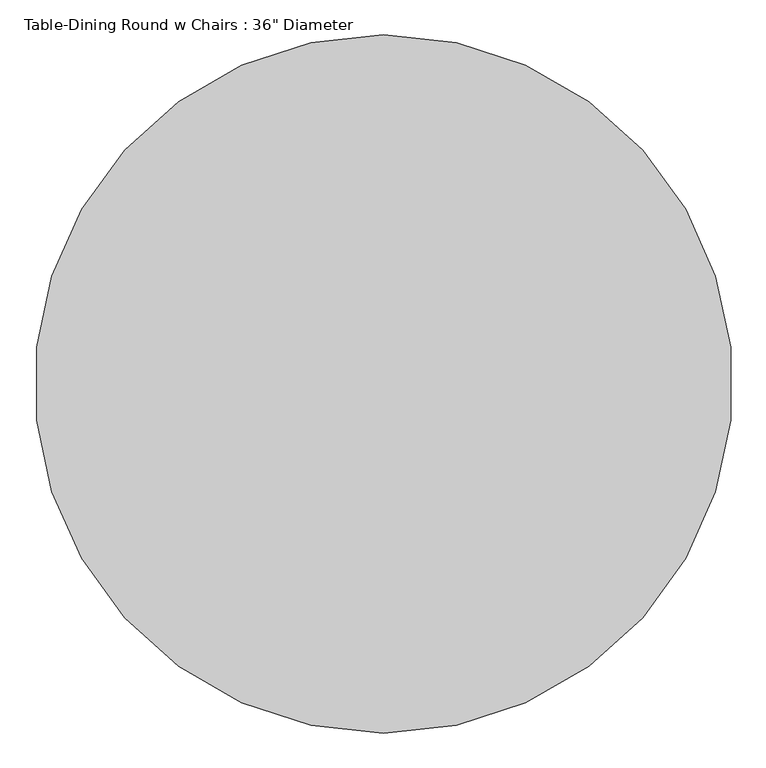
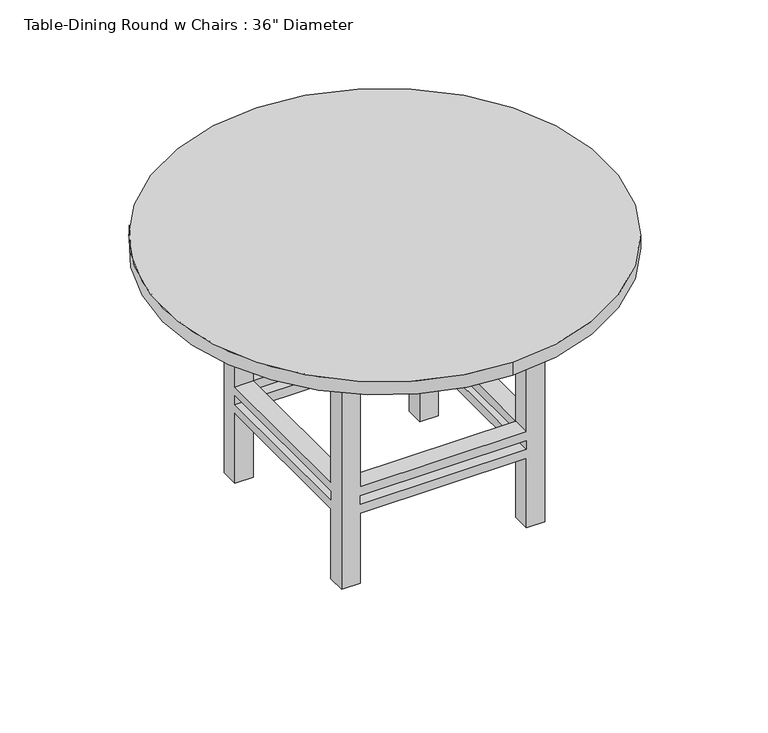
"""IFC4 building model written with IfcOpenShell, lengths in millimetres: furniture geometry."""

from ifc_helpers import new_model, si_unit, point, frame, frame_2d, origin, place, context, project, spatial, polyline, circle_curve, trimmed, segment, composite_curve, outline, extrude, faceted_brep, source, transform, mapped, element, save


def furniture_7060ebe6(model_context):
    return source(origin(), model_context, "Body", "SolidModel", [
        faceted_brep([(332.2819672, 43.7213115, 279.4), (332.2819672, -413.4786885, 279.4), (383.0819672, -413.4786885, 279.4), (383.0819672, 43.7213115, 279.4), (-124.9180328, -413.4786885, 279.4), (-124.9180328, -464.2786885, 279.4), (332.2819672, -464.2786885, 279.4), (-124.9180328, 43.7213115, 279.4), (-175.7180328, 43.7213115, 279.4), (-175.7180328, -413.4786885, 279.4), (332.2819672, 94.5213115, 279.4), (-124.9180328, 94.5213115, 279.4), (332.2819672, 43.7213115, 254.0), (-124.9180328, 43.7213115, 254.0), (-124.9180328, 94.5213115, 254.0), (332.2819672, 94.5213115, 254.0), (-124.9180328, -413.4786885, 254.0), (-175.7180328, -413.4786885, 254.0), (-175.7180328, 43.7213115, 254.0), (332.2819672, -413.4786885, 254.0), (332.2819672, -464.2786885, 254.0), (-124.9180328, -464.2786885, 254.0), (383.0819672, 43.7213115, 254.0), (383.0819672, -413.4786885, 254.0), (-175.7180328, 94.5213115, 647.7), (-124.9180328, 94.5213115, 647.7), (332.2819672, 94.5213115, 647.7), (383.0819672, 94.5213115, 647.7), (383.0819672, 94.5213115, 0.0), (332.2819672, 94.5213115, 0.0), (332.2819672, 94.5213115, 203.2), (-124.9180328, 94.5213115, 203.2), (-124.9180328, 94.5213115, 0.0), (-175.7180328, 94.5213115, 0.0), (-124.9180328, 94.5213115, 228.6), (332.2819672, 94.5213115, 228.6), (-175.7180328, 43.7213115, 647.7), (-175.7180328, 43.7213115, 0.0), (-175.7180328, 43.7213115, 203.2), (-175.7180328, -413.4786885, 203.2), (-175.7180328, -413.4786885, 0.0), (-175.7180328, -464.2786885, 0.0), (-175.7180328, -464.2786885, 647.7), (-175.7180328, -413.4786885, 647.7), (-175.7180328, -413.4786885, 228.6), (-175.7180328, 43.7213115, 228.6), (383.0819672, -464.2786885, 647.7), (332.2819672, -464.2786885, 647.7), (-124.9180328, -464.2786885, 647.7), (-124.9180328, -464.2786885, 0.0), (-124.9180328, -464.2786885, 203.2), (332.2819672, -464.2786885, 203.2), (332.2819672, -464.2786885, 0.0), (383.0819672, -464.2786885, 0.0), (332.2819672, -464.2786885, 228.6), (-124.9180328, -464.2786885, 228.6), (383.0819672, 43.7213115, 647.7), (383.0819672, -413.4786885, 647.7), (383.0819672, -413.4786885, 0.0), (383.0819672, -413.4786885, 203.2), (383.0819672, 43.7213115, 203.2), (383.0819672, 43.7213115, 0.0), (383.0819672, 43.7213115, 228.6), (383.0819672, -413.4786885, 228.6), (-124.9180328, 43.7213115, 647.7), (332.2819672, -413.4786885, 647.7), (332.2819672, 43.7213115, 647.7), (-124.9180328, -413.4786885, 647.7), (332.2819672, 43.7213115, 0.0), (-124.9180328, -413.4786885, 0.0), (-124.9180328, 43.7213115, 0.0), (332.2819672, -413.4786885, 0.0), (-124.9180328, 43.7213115, 228.6), (-124.9180328, 43.7213115, 203.2), (332.2819672, 43.7213115, 228.6), (332.2819672, 43.7213115, 203.2), (332.2819672, -413.4786885, 228.6), (332.2819672, -413.4786885, 203.2), (-124.9180328, -413.4786885, 228.6), (-124.9180328, -413.4786885, 203.2)], [[[0, 1, 2, 3]], [[1, 4, 5, 6]], [[4, 7, 8, 9]], [[7, 0, 10, 11]], [[12, 13, 14, 15]], [[13, 16, 17, 18]], [[16, 19, 20, 21]], [[19, 12, 22, 23]], [[24, 25, 11, 10, 26, 27, 28, 29, 30, 31, 32, 33], [14, 34, 35, 15]], [[36, 24, 33, 37, 38, 39, 40, 41, 42, 43, 9, 8], [17, 44, 45, 18]], [[46, 47, 6, 5, 48, 42, 41, 49, 50, 51, 52, 53], [20, 54, 55, 21]], [[28, 27, 56, 3, 2, 57, 46, 53, 58, 59, 60, 61], [22, 62, 63, 23]], [[1, 0, 12, 19]], [[4, 1, 19, 16]], [[7, 4, 16, 13]], [[0, 7, 13, 12]], [[25, 24, 36, 64]], [[47, 46, 57, 65]], [[26, 66, 56, 27]], [[48, 67, 43, 42]], [[29, 28, 61, 68]], [[49, 41, 40, 69]], [[32, 70, 37, 33]], [[52, 71, 58, 53]], [[13, 18, 45, 72]], [[64, 36, 8, 7]], [[37, 70, 73, 38]], [[14, 13, 72, 34]], [[25, 64, 7, 11]], [[70, 32, 31, 73]], [[12, 15, 35, 74]], [[66, 26, 10, 0]], [[29, 68, 75, 30]], [[22, 12, 74, 62]], [[56, 66, 0, 3]], [[68, 61, 60, 75]], [[19, 23, 63, 76]], [[65, 57, 2, 1]], [[58, 71, 77, 59]], [[20, 19, 76, 54]], [[47, 65, 1, 6]], [[71, 52, 51, 77]], [[16, 21, 55, 78]], [[67, 48, 5, 4]], [[49, 69, 79, 50]], [[17, 16, 78, 44]], [[43, 67, 4, 9]], [[69, 40, 39, 79]], [[74, 76, 63, 62]], [[76, 78, 55, 54]], [[78, 72, 45, 44]], [[72, 74, 35, 34]], [[75, 73, 31, 30]], [[73, 79, 39, 38]], [[79, 77, 51, 50]], [[77, 75, 60, 59]], [[76, 74, 75, 77]], [[78, 76, 77, 79]], [[72, 78, 79, 73]], [[74, 72, 73, 75]]]),
        extrude(outline(polyline([(408.4819672, 119.9213115), (408.4819672, -489.6786885), (-201.1180328, -489.6786885), (-201.1180328, 119.9213115), (408.4819672, 119.9213115)]), holes=[polyline([(383.0819672, 94.5213115), (-175.7180328, 94.5213115), (-175.7180328, -464.2786885), (383.0819672, -464.2786885), (383.0819672, 94.5213115)])]), frame((0.0, 0.0, 647.7), z_axis=(0.0, 0.0, 1.0), x_axis=(1.0, 0.0, 0.0)), (0.0, 0.0, 1.0), 76.2),
        extrude(outline(composite_curve([segment(trimmed(circle_curve(frame_2d((103.6819672, -184.8786885)), 609.6), [point((103.6819672, -794.4786885))], [point((103.6819672, 424.7213115))], False, "CARTESIAN"), True, "CONTINUOUS"), segment(trimmed(circle_curve(frame_2d((103.6819672, -184.8786885)), 609.6), [point((103.6819672, 424.7213115))], [point((103.6819672, -794.4786885))], False, "CARTESIAN"), True, "CONTINUOUS")], self_intersect=False)), frame((0.0, 0.0, 723.9), z_axis=(0.0, 0.0, 1.0), x_axis=(1.0, 0.0, 0.0)), (0.0, 0.0, 1.0), 38.1),
    ])


if __name__ == "__main__":
    model = new_model("IFC4")
    model_context = context("Model", 3, world=origin())
    ifc_project = project(units=[si_unit("LENGTHUNIT", "METRE", prefix="MILLI")], contexts=[model_context])
    site = spatial("IfcSite", under=ifc_project)
    building = spatial("IfcBuilding", under=site)
    placement = place(None, origin())
    furniture_shape = furniture_7060ebe6(model_context)
    element("IfcFurniture", 1, ObjectType="Table-Dining Round w Chairs : 36\" Diameter", at=placement, inside=building, context=model_context, shape_type="MappedRepresentation", body=[
        mapped(furniture_shape, transform((0.0, 0.0, 0.0), x_axis=(1.0, 0.0, 0.0), y_axis=(0.0, 1.0, 0.0), z_axis=(0.0, 0.0, 1.0))),
    ])
    save(model, "model.ifc")

# Revit data of these elements
# Type "Table-Dining Round w Chairs : 36\" Diameter"
#   Assembly Code = "E2020200"
#   Radius = 2' - 0"
#   Diameter = 4' - 0"
#   Height = 2' - 6"
#   Chairs = 6
#   Base Material = Pine
#   Top Material = Laminate, Linen, Matte
#   Default Elevation = 0
# Element 1 (IfcFurniture, "Table-Dining Round w Chairs : 36\" Diameter")
#   Materials on its faces: "Pine", "Laminate, Linen, Matte"
# Materials
#   "Pine": class "Wood", colour RGB 223 192 134, transparency 0, Description = "Pinus Echinata", Cost = 0
#   "Laminate, Linen, Matte": class "Plastic", colour RGB 249 239 230, transparency 0, Description = "Plastic Laminate - Linen, Matte", Cost = 0
